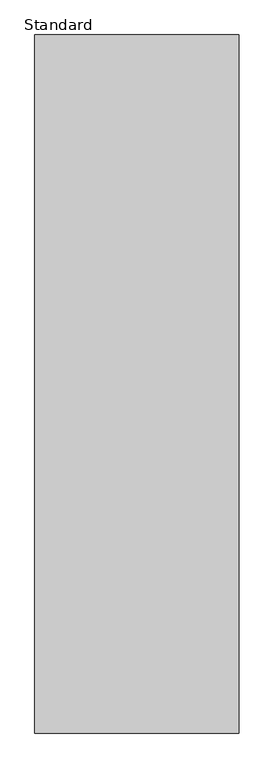
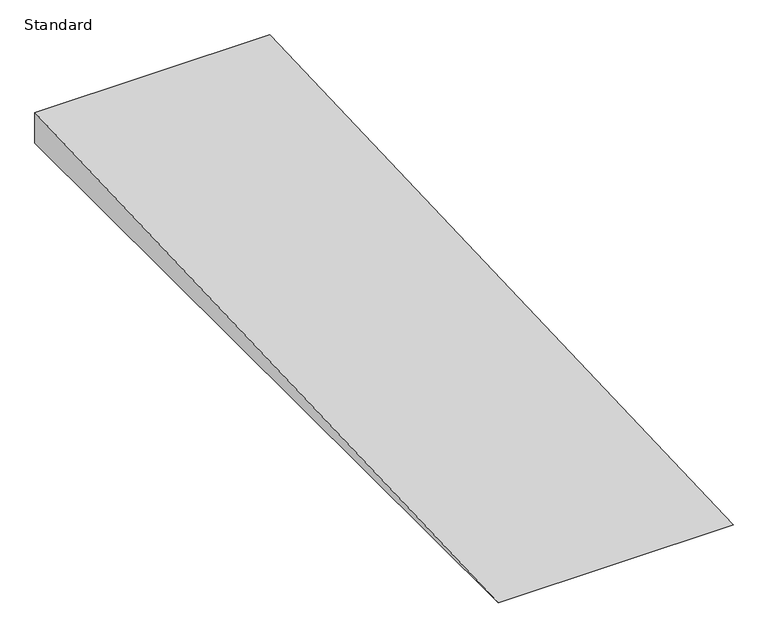
"""IFC4 building model written with IfcOpenShell, lengths in millimetres: ramp geometry, Standard."""

from ifc_helpers import new_model, si_unit, frame, origin, place, context, project, spatial, polyline, outline, extrude, source, transform, mapped, element, save


def standard_832cbf63(model_context):
    return source(origin(), model_context, "Body", "SweptSolid", [
        extrude(outline(polyline([(-14223.0543293, 0.0), (-520.8977554, 548.086263), (-520.8977554, 0.0), (-14223.0543293, 0.0)])), frame((-13246.6151539, 0.0, 0.0), z_axis=(1.0, 0.0, 0.0), x_axis=(0.0, 1.0, 0.0)), (0.0, 0.0, 1.0), 4013.2),
    ])


if __name__ == "__main__":
    model = new_model("IFC4")
    model_context = context("Model", 3, world=origin())
    ifc_project = project(units=[si_unit("LENGTHUNIT", "METRE", prefix="MILLI")], contexts=[model_context])
    site = spatial("IfcSite", under=ifc_project)
    building = spatial("IfcBuilding", under=site)
    placement = place(None, origin())
    standard_shape = standard_832cbf63(model_context)
    element("IfcRamp", 1, ObjectType="Standard", at=placement, inside=building, context=model_context, shape_type="MappedRepresentation", body=[
        mapped(standard_shape, transform((0.0, 0.0, 0.0), x_axis=(1.0, 0.0, 0.0), y_axis=(0.0, 1.0, 0.0), z_axis=(0.0, 0.0, 1.0))),
    ])
    save(model, "model.ifc")
